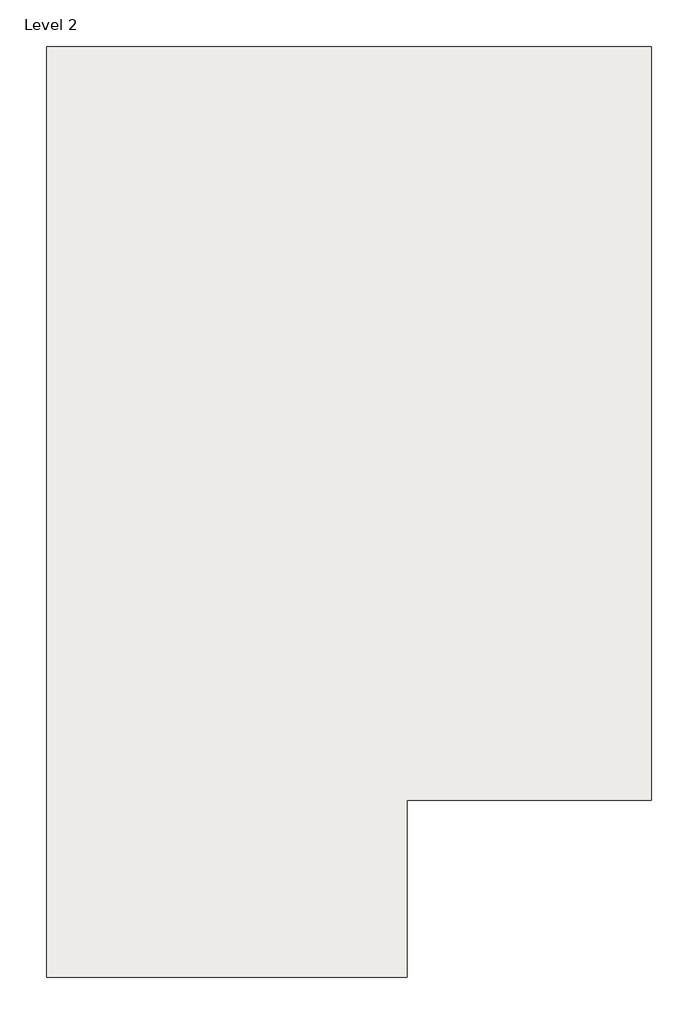
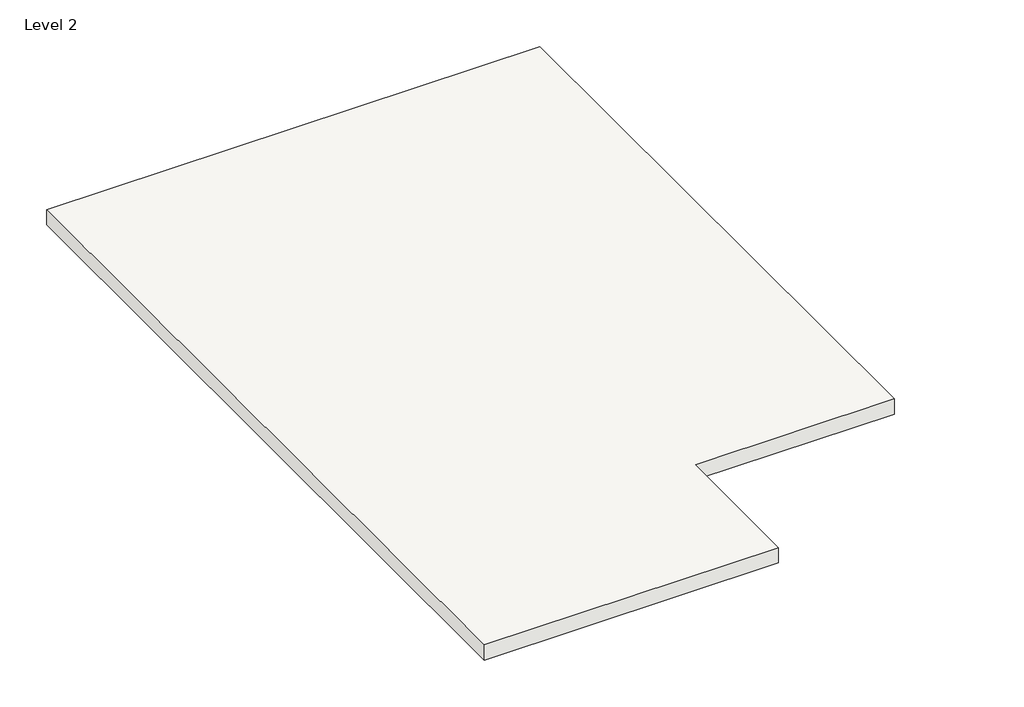
# One storey: 1 roof.
"""IFC4 building model written with IfcOpenShell, lengths in millimetres."""

from ifc_helpers import new_model, si_unit, frame, origin, place, context, project, spatial, polyline, outline, extrude, element, save

model = new_model("IFC4")

# Units and contexts
model_context = context("Model", 3, world=origin())
ifc_project = project(units=[si_unit("LENGTHUNIT", "METRE", prefix="MILLI")], contexts=[model_context])

# Site, building, storey
site = spatial("IfcSite", under=ifc_project)
building = spatial("IfcBuilding", under=site)
storey = spatial("IfcBuildingStorey", under=building, Name="Level 2", Elevation=3048.0)

# Roof
placement = place(None, origin())
element("IfcRoof", 1, ObjectType="Generic - 12\"", at=placement, inside=storey, context=model_context, shape_type="SweptSolid", body=[
    extrude(outline(polyline([(-14558.7660538, 14369.953629), (-5186.1660538, 14369.953629), (-5186.1660538, 2692.303629), (-8970.7660538, 2692.303629), (-8970.7660538, -50.896371), (-14558.7660538, -50.896371), (-14558.7660538, 14369.953629)])), frame((0.0, 0.0, 3048.0), z_axis=(0.0, 0.0, 1.0), x_axis=(1.0, 0.0, 0.0)), (0.0, 0.0, 1.0), 304.8),
])

save(model, "model.ifc")

# Revit data of these elements
# Type "Generic - 12\""
#   Assembly Code = "B1020"
#   Layers, outside or top first: 1' - 0" "Brick, Soldier Course" (function 1)
# Element 1 (IfcRoof, "Generic - 12\"")
#   built-in parameter 1001705 = 11 (stored number, unit not read)
#   built-in parameter 1001710 = 33615
#   Phase Created = New Construction
#   Materials on its faces: "Brick, Soldier Course"
# Materials
#   "Brick, Soldier Course": class "Masonry", colour RGB 170 98 104, transparency 0, Description = "Common brick soldier coursed", Cost = 0
